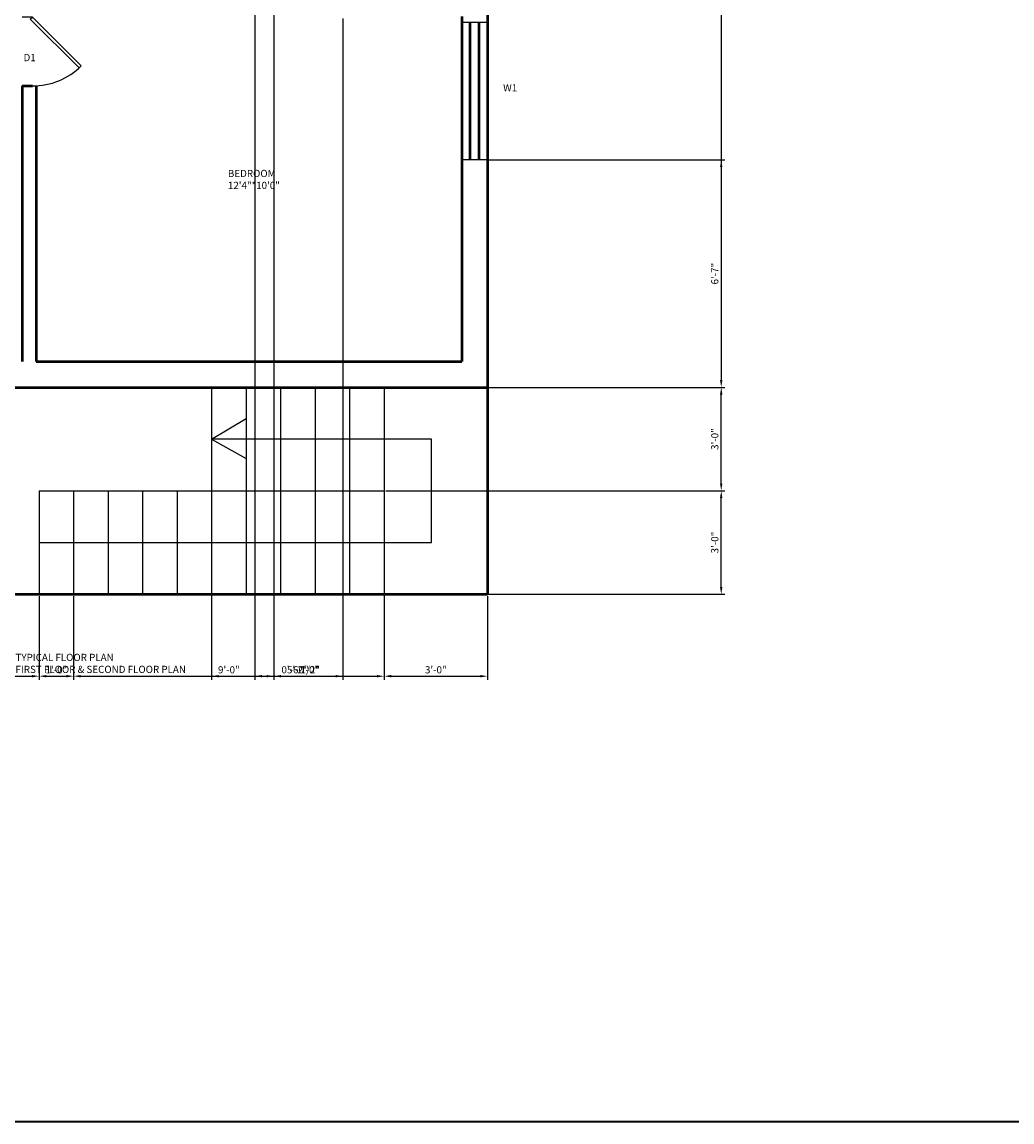
# Model space of a CAD drawing. Units: inches. Extents: x 2020 to 7901, y 1581 to 3943.
# Tile 10 of 17: x 3141 to 3486, y 1581 to 1963. Entities that reach past the tile are written whole.
import ezdxf

# ---------------------------------------------------------------- set-up
doc = ezdxf.new("R2010")
doc.units = ezdxf.units.IN
for name, color, linetype, lineweight in [('A-ANNO-DIMS', 2, 'Continuous', 18), ('A-ANNO-TEXT', 7, 'Continuous', 18), ('A-ANNO-TTLB', 7, 'Continuous', 35), ('A-AREA-IDEN', 3, 'Continuous', 18), ('A-DOOR', 4, 'Continuous', 25), ('A-FLOR-STRS', 3, 'Continuous', 25), ('A-GLAZ', 4, 'Continuous', 25), ('A-WALL', 7, 'Continuous', 50)]:
    doc.layers.add(name, color=color, linetype=linetype, lineweight=lineweight)
doc.styles.get("Standard").update_dxf_attribs({"font": 'arial.ttf'})
doc.dimstyles.new('ISO-25', dxfattribs={"dimtxt": 2.5, "dimasz": 2.5, "dimexe": 1.25, "dimexo": 0.625, "dimtad": 1, "dimdec": 1, "dimlunit": 3, "dimtxsty": 'Standard', "dimcen": 2.5, "dimadec": 0, "dimazin": 0, "dimtfac": 1, "dimtdec": 1, "dimtmove": 0, "dimatfit": 3, "dimfxl": 1, "dimarcsym": 0})

# ---------------------------------------------------------------- blocks, each defined once
blk = doc.blocks.new('*U10')
for p, q in [((0, 0), (0, -6)), ((40, 0), (40, -6))]:
    blk.add_line(p, q)
blk.add_lwpolyline([(0, 0), (28.28, 28.28), (29.52, 27.05), (1.24, -1.24)], close=True)
blk.add_arc((0, 0), 40, 0, 45)
blk = doc.blocks.new('WIN-1200')
for p, q in [((0, 9), (48, 9)), ((0, 0), (0, 9)), ((48, 9), (48, 0)), ((48, 0), (0, 0))]:
    blk.add_line(p, q)
blk = doc.blocks.new('*D50')
at = {"layer": 'A-ANNO-DIMS', "color": 0, "lineweight": -2, "transparency": 16777216}
for p, q in [((3303.94, 1915.45), (3385.87, 1915.45)), ((3384.62, 1912.95), (3384.62, 1838.84)), ((3303.94, 1836.34), (3385.87, 1836.34))]:
    blk.add_line(p, q, dxfattribs=at)
at = {"layer": 'A-ANNO-DIMS', "color": 0, "transparency": 16777216}
for points in [[(3384.2, 1912.95), (3385.03, 1912.95), (3384.62, 1915.45)], [(3384.2, 1838.84), (3385.03, 1838.84), (3384.62, 1836.34)]]:
    blk.add_solid(points, dxfattribs=at)
at = {"layer": 'DEFPOINTS', "color": 0, "transparency": 16777216}
for p in [(3303.32, 1915.45), (3303.32, 1836.34), (3384.62, 1836.34)]:
    blk.add_point(p, dxfattribs=at)
at = {"layer": 'A-ANNO-DIMS', "color": 0, "transparency": 16777216, "insert": (3382.71, 1875.9), "char_height": 2.5, "attachment_point": 5, "rotation": 90}
blk.add_mtext('6\'-7"', dxfattribs=at)
blk = doc.blocks.new('*D51')
at = {"layer": 'A-ANNO-DIMS', "color": 0, "lineweight": -2, "transparency": 16777216}
for p, q in [((2970.32, 1763.71), (2970.32, 1734.59)), ((3147.32, 1763.71), (3147.32, 1734.59)), ((2972.82, 1735.84), (3144.82, 1735.84))]:
    blk.add_line(p, q, dxfattribs=at)
at = {"layer": 'A-ANNO-DIMS', "color": 0, "transparency": 16777216}
for points in [[(2972.82, 1736.26), (2972.82, 1735.42), (2970.32, 1735.84)], [(3144.82, 1736.26), (3144.82, 1735.42), (3147.32, 1735.84)]]:
    blk.add_solid(points, dxfattribs=at)
at = {"layer": 'DEFPOINTS', "color": 0, "transparency": 16777216}
for p in [(2970.32, 1764.34), (3147.32, 1764.34), (3147.32, 1735.84)]:
    blk.add_point(p, dxfattribs=at)
at = {"layer": 'A-ANNO-DIMS', "color": 0, "transparency": 16777216, "insert": (3058.82, 1737.74), "char_height": 2.5, "attachment_point": 5}
blk.add_mtext('14\'-9"', dxfattribs=at)
blk = doc.blocks.new('*D52')
at = {"layer": 'A-ANNO-DIMS', "color": 0, "lineweight": -2, "transparency": 16777216}
for p, q in [((3147.32, 1763.71), (3147.32, 1734.59)), ((3159.32, 1763.71), (3159.32, 1734.59)), ((3149.82, 1735.84), (3156.82, 1735.84))]:
    blk.add_line(p, q, dxfattribs=at)
at = {"layer": 'A-ANNO-DIMS', "color": 0, "transparency": 16777216}
for points in [[(3149.82, 1736.26), (3149.82, 1735.42), (3147.32, 1735.84)], [(3156.82, 1736.26), (3156.82, 1735.42), (3159.32, 1735.84)]]:
    blk.add_solid(points, dxfattribs=at)
at = {"layer": 'DEFPOINTS', "color": 0, "transparency": 16777216}
for p in [(3147.32, 1764.34), (3159.32, 1764.34), (3159.32, 1735.84)]:
    blk.add_point(p, dxfattribs=at)
at = {"layer": 'A-ANNO-DIMS', "color": 0, "transparency": 16777216, "insert": (3153.32, 1737.74), "char_height": 2.5, "attachment_point": 5}
blk.add_mtext('1\'-0"', dxfattribs=at)
blk = doc.blocks.new('*D53')
at = {"layer": 'A-ANNO-DIMS', "color": 0, "lineweight": -2, "transparency": 16777216}
for p, q in [((3159.32, 1763.71), (3159.32, 1734.59)), ((3267.32, 1763.71), (3267.32, 1734.59)), ((3161.82, 1735.84), (3264.82, 1735.84))]:
    blk.add_line(p, q, dxfattribs=at)
at = {"layer": 'A-ANNO-DIMS', "color": 0, "transparency": 16777216}
for points in [[(3161.82, 1736.26), (3161.82, 1735.42), (3159.32, 1735.84)], [(3264.82, 1736.26), (3264.82, 1735.42), (3267.32, 1735.84)]]:
    blk.add_solid(points, dxfattribs=at)
at = {"layer": 'DEFPOINTS', "color": 0, "transparency": 16777216}
for p in [(3159.32, 1764.34), (3267.32, 1764.34), (3267.32, 1735.84)]:
    blk.add_point(p, dxfattribs=at)
at = {"layer": 'A-ANNO-DIMS', "color": 0, "transparency": 16777216, "insert": (3213.32, 1737.74), "char_height": 2.5, "attachment_point": 5}
blk.add_mtext('9\'-0"', dxfattribs=at)
blk = doc.blocks.new('*D54')
at = {"layer": 'A-ANNO-DIMS', "color": 0, "lineweight": -2, "transparency": 16777216}
for p, q in [((3267.32, 1763.71), (3267.32, 1734.59)), ((3303.32, 1763.71), (3303.32, 1734.59)), ((3269.82, 1735.84), (3300.82, 1735.84))]:
    blk.add_line(p, q, dxfattribs=at)
at = {"layer": 'A-ANNO-DIMS', "color": 0, "transparency": 16777216}
for points in [[(3269.82, 1736.26), (3269.82, 1735.42), (3267.32, 1735.84)], [(3300.82, 1736.26), (3300.82, 1735.42), (3303.32, 1735.84)]]:
    blk.add_solid(points, dxfattribs=at)
at = {"layer": 'DEFPOINTS', "color": 0, "transparency": 16777216}
for p in [(3267.32, 1764.34), (3303.32, 1764.34), (3303.32, 1735.84)]:
    blk.add_point(p, dxfattribs=at)
at = {"layer": 'A-ANNO-DIMS', "color": 0, "transparency": 16777216, "insert": (3285.32, 1737.74), "char_height": 2.5, "attachment_point": 5}
blk.add_mtext('3\'-0"', dxfattribs=at)
blk = doc.blocks.new('*D56')
at = {"layer": 'A-ANNO-DIMS', "color": 0, "lineweight": -2, "transparency": 16777216}
for p, q in [((3267.94, 1800.34), (3385.87, 1800.34)), ((3384.62, 1766.84), (3384.62, 1797.84)), ((3267.94, 1764.34), (3385.87, 1764.34))]:
    blk.add_line(p, q, dxfattribs=at)
at = {"layer": 'A-ANNO-DIMS', "color": 0, "transparency": 16777216}
for points in [[(3384.2, 1797.84), (3385.03, 1797.84), (3384.62, 1800.34)], [(3384.2, 1766.84), (3385.03, 1766.84), (3384.62, 1764.34)]]:
    blk.add_solid(points, dxfattribs=at)
at = {"layer": 'DEFPOINTS', "color": 0, "transparency": 16777216}
for p in [(3267.32, 1800.34), (3384.62, 1800.34), (3267.32, 1764.34)]:
    blk.add_point(p, dxfattribs=at)
at = {"layer": 'A-ANNO-DIMS', "color": 0, "transparency": 16777216, "insert": (3382.71, 1782.34), "char_height": 2.5, "attachment_point": 5, "rotation": 90}
blk.add_mtext('3\'-0"', dxfattribs=at)
blk = doc.blocks.new('*D123')
at = {"layer": 'A-ANNO-DIMS', "color": 0, "lineweight": -2, "transparency": 16777216}
for p, q in [((3303.94, 2214.34), (3385.87, 2214.34)), ((3384.62, 2211.84), (3384.62, 1838.84)), ((3303.94, 1836.34), (3385.87, 1836.34))]:
    blk.add_line(p, q, dxfattribs=at)
at = {"layer": 'A-ANNO-DIMS', "color": 0, "transparency": 16777216}
for points in [[(3384.2, 2211.84), (3385.03, 2211.84), (3384.62, 2214.34)], [(3384.2, 1838.84), (3385.03, 1838.84), (3384.62, 1836.34)]]:
    blk.add_solid(points, dxfattribs=at)
at = {"layer": 'DEFPOINTS', "color": 0, "transparency": 16777216}
for p in [(3303.32, 2214.34), (3303.32, 1836.34), (3384.62, 1836.34)]:
    blk.add_point(p, dxfattribs=at)
at = {"layer": 'A-ANNO-DIMS', "color": 0, "transparency": 16777216, "insert": (3382.71, 2025.34), "char_height": 2.5, "attachment_point": 5, "rotation": 90}
blk.add_mtext('31\'-6"', dxfattribs=at)
blk = doc.blocks.new('*D136')
at = {"layer": 'A-ANNO-DIMS', "color": 0, "lineweight": -2, "transparency": 16777216}
for p, q in [((3222.32, 1969.71), (3222.32, 1734.59)), ((3228.97, 1969.71), (3228.97, 1734.59)), ((3224.82, 1735.84), (3226.47, 1735.84)), ((3228.97, 1735.84), (3245.19, 1735.84))]:
    blk.add_line(p, q, dxfattribs=at)
at = {"layer": 'A-ANNO-DIMS', "color": 0, "transparency": 16777216}
for points in [[(3224.82, 1736.26), (3224.82, 1735.42), (3222.32, 1735.84)], [(3226.47, 1736.26), (3226.47, 1735.42), (3228.97, 1735.84)]]:
    blk.add_solid(points, dxfattribs=at)
at = {"layer": 'DEFPOINTS', "color": 0, "transparency": 16777216}
for p in [(3222.32, 1970.34), (3228.97, 1970.34), (3228.97, 1735.84)]:
    blk.add_point(p, dxfattribs=at)
at = {"layer": 'A-ANNO-DIMS', "color": 0, "transparency": 16777216, "insert": (3238.33, 1737.76), "char_height": 2.5, "attachment_point": 5}
blk.add_mtext('0\'-6 1/2"', dxfattribs=at)
blk = doc.blocks.new('*D137')
at = {"layer": 'A-ANNO-DIMS', "color": 0, "lineweight": -2, "transparency": 16777216}
for p, q in [((3228.97, 1964.72), (3228.97, 1734.59)), ((3252.97, 1964.72), (3252.97, 1734.59)), ((3231.47, 1735.84), (3250.47, 1735.84))]:
    blk.add_line(p, q, dxfattribs=at)
at = {"layer": 'A-ANNO-DIMS', "color": 0, "transparency": 16777216}
for points in [[(3231.47, 1736.26), (3231.47, 1735.42), (3228.97, 1735.84)], [(3250.47, 1736.26), (3250.47, 1735.42), (3252.97, 1735.84)]]:
    blk.add_solid(points, dxfattribs=at)
at = {"layer": 'DEFPOINTS', "color": 0, "transparency": 16777216}
for p in [(3228.97, 1965.35), (3252.97, 1965.35), (3252.97, 1735.84)]:
    blk.add_point(p, dxfattribs=at)
at = {"layer": 'A-ANNO-DIMS', "color": 0, "transparency": 16777216, "insert": (3240.97, 1737.74), "char_height": 2.5, "attachment_point": 5}
blk.add_mtext('2\'-0"', dxfattribs=at)
blk = doc.blocks.new('*D145')
at = {"layer": 'A-ANNO-DIMS', "color": 0, "lineweight": -2, "transparency": 16777216}
for p, q in [((3207.32, 1835.71), (3207.32, 1734.59)), ((3267.32, 1835.71), (3267.32, 1734.59)), ((3209.82, 1735.84), (3264.82, 1735.84))]:
    blk.add_line(p, q, dxfattribs=at)
at = {"layer": 'A-ANNO-DIMS', "color": 0, "transparency": 16777216}
for points in [[(3209.82, 1736.26), (3209.82, 1735.42), (3207.32, 1735.84)], [(3264.82, 1736.26), (3264.82, 1735.42), (3267.32, 1735.84)]]:
    blk.add_solid(points, dxfattribs=at)
at = {"layer": 'DEFPOINTS', "color": 0, "transparency": 16777216}
for p in [(3207.32, 1836.34), (3267.32, 1836.34), (3267.32, 1735.84)]:
    blk.add_point(p, dxfattribs=at)
at = {"layer": 'A-ANNO-DIMS', "color": 0, "transparency": 16777216, "insert": (3237.32, 1737.74), "char_height": 2.5, "attachment_point": 5}
blk.add_mtext('5\'-0"', dxfattribs=at)
blk = doc.blocks.new('*D146')
at = {"layer": 'A-ANNO-DIMS', "color": 0, "lineweight": -2, "transparency": 16777216}
for p, q in [((3267.94, 1836.34), (3385.87, 1836.34)), ((3384.62, 1802.84), (3384.62, 1833.84)), ((3267.94, 1800.34), (3385.87, 1800.34))]:
    blk.add_line(p, q, dxfattribs=at)
at = {"layer": 'A-ANNO-DIMS', "color": 0, "transparency": 16777216}
for points in [[(3384.2, 1833.84), (3385.03, 1833.84), (3384.62, 1836.34)], [(3384.2, 1802.84), (3385.03, 1802.84), (3384.62, 1800.34)]]:
    blk.add_solid(points, dxfattribs=at)
at = {"layer": 'DEFPOINTS', "color": 0, "transparency": 16777216}
for p in [(3267.32, 1836.34), (3384.62, 1836.34), (3267.32, 1800.34)]:
    blk.add_point(p, dxfattribs=at)
at = {"layer": 'A-ANNO-DIMS', "color": 0, "transparency": 16777216, "insert": (3382.71, 1818.34), "char_height": 2.5, "attachment_point": 5, "rotation": 90}
blk.add_mtext('3\'-0"', dxfattribs=at)

msp = doc.modelspace()

# ---------------------------------------------------------------- linework, layer by layer
at = {"layer": 'A-ANNO-TTLB'}
msp.add_lwpolyline([(2019.8, 3067.25), (4199.03, 3067.25), (4199.03, 1580.73), (2019.8, 1580.73)], close=True, dxfattribs=at)
at = {"layer": 'A-FLOR-STRS'}
for p, q in [((3207.32, 1836.34), (3207.32, 1764.34)), ((3219.32, 1836.34), (3219.32, 1764.34)), ((3231.32, 1836.34), (3231.32, 1764.34)), ((3243.32, 1836.34), (3243.32, 1764.34)), ((3255.32, 1836.34), (3255.32, 1764.34)), ((3267.32, 1836.34), (3267.32, 1764.34)), ((3207.32, 1818.34), (3219.32, 1825.47)), ((3283.87, 1818.34), (3207.32, 1818.34)), ((3207.32, 1818.34), (3219.32, 1811.61)), ((3283.87, 1782.34), (3283.87, 1818.34)), ((3147.32, 1800.34), (3147.32, 1764.34)), ((3147.32, 1800.34), (3267.32, 1800.34)), ((3159.32, 1800.34), (3159.32, 1764.34)), ((3171.32, 1800.34), (3171.32, 1764.34)), ((3183.32, 1800.34), (3183.32, 1764.34)), ((3195.32, 1800.34), (3195.32, 1764.34)), ((3147.32, 1782.34), (3283.87, 1782.34))]:
    msp.add_line(p, q, dxfattribs=at)
at = {"layer": 'A-WALL'}
for p, q in [((3303.32, 2240.34), (3303.32, 1764.34)), ((3294.32, 1965.34), (3294.32, 1845.34)), ((3297.32, 1915.45), (3297.32, 1963.45)), ((3300.32, 1963.45), (3300.32, 1915.45)), ((3141.39, 1941.19), (3144.99, 1941.19)), ((3141.39, 1941.19), (3141.39, 1845.34)), ((3146.32, 1941.23), (3146.32, 1845.34)), ((3146.32, 1845.34), (3294.32, 1845.34)), ((3061.63, 1836.34), (3303.32, 1836.34)), ((2970.32, 1764.34), (3303.32, 1764.34))]:
    msp.add_line(p, q, dxfattribs=at)

# ---------------------------------------------------------------- block references
at = {"layer": 'A-DOOR', "xscale": 0.6, "yscale": 0.6, "zscale": 0.6, "rotation": 270}
msp.add_blockref('*U10', (3144.99, 1965.19), dxfattribs=at)
at = {"layer": 'A-GLAZ', "rotation": 89.999999999998}
msp.add_blockref('WIN-1200', (3303.32, 1915.45), dxfattribs=at)

# ---------------------------------------------------------------- texts
at = {"layer": 'A-ANNO-TEXT', "char_height": 2.5, "attachment_point": 1}
for s, width, insert in [('D1', 8.3071, (3141.91, 1952.32)), ('W1', 12.448, (3308.75, 1941.8)), ('TYPICAL FLOOR PLAN\\PFIRST FLOOR & SECOND FLOOR PLAN', 248.2469, (3139.1, 1743.63))]:
    msp.add_mtext_dynamic_manual_height_columns(s, width=width, gutter_width=12.5, heights=[0], dxfattribs=dict(at, insert=insert))
at = {"layer": 'A-AREA-IDEN', "insert": (3212.99, 1912.01), "char_height": 2.5, "attachment_point": 1}
msp.add_mtext_dynamic_manual_height_columns('BEDROOM\\P12\'4"*10\'0"', width=79.8865, gutter_width=12.5, heights=[0], dxfattribs=at)

# ---------------------------------------------------------------- dimensions: what is measured, and where the dimension line sits
at = {"layer": 'A-ANNO-DIMS'}
for base, p1, p2, picture, middle in [((3384.62, 1836.34), (3303.32, 2214.34), (3303.32, 1836.34), '*D123', (3382.71, 2025.34)), ((3384.62, 1836.34), (3303.32, 1915.45), (3303.32, 1836.34), '*D50', (3382.71, 1875.9)), ((3384.62, 1836.34), (3267.32, 1800.34), (3267.32, 1836.34), '*D146', (3382.71, 1818.34)), ((3384.62, 1800.34), (3267.32, 1764.34), (3267.32, 1800.34), '*D56', (3382.71, 1782.34))]:
    dim = msp.add_linear_dim(base=base, p1=p1, p2=p2, angle=90, dimstyle='ISO-25', override={"dimdec": 1, "dimlfac": 1, "dimrnd": 0, "dimzin": 1, "dimdsep": 46, "dimlunit": 4, "dimfrac": 2}, dxfattribs=at)
    dim.commit()
    dim.dimension.update_dxf_attribs({"geometry": picture, "text_midpoint": middle})
for base, p1, p2, picture, middle in [((3228.9718, 1735.8394), (3222.3165, 1970.3394), (3228.9718, 1970.3394), '*D136', (3238.3323, 1737.7571)), ((3252.97, 1735.84), (3228.97, 1965.35), (3252.97, 1965.35), '*D137', (3240.97, 1737.74)), ((3267.32, 1735.84), (3207.32, 1836.34), (3267.32, 1836.34), '*D145', (3237.32, 1737.74)), ((3147.32, 1735.84), (2970.32, 1764.34), (3147.32, 1764.34), '*D51', (3058.82, 1737.74)), ((3159.32, 1735.84), (3147.32, 1764.34), (3159.32, 1764.34), '*D52', (3153.32, 1737.74)), ((3267.32, 1735.84), (3159.32, 1764.34), (3267.32, 1764.34), '*D53', (3213.32, 1737.74)), ((3303.32, 1735.84), (3267.32, 1764.34), (3303.32, 1764.34), '*D54', (3285.32, 1737.74))]:
    dim = msp.add_linear_dim(base=base, p1=p1, p2=p2, dimstyle='ISO-25', override={"dimdec": 1, "dimlfac": 1, "dimrnd": 0, "dimzin": 1, "dimdsep": 46, "dimlunit": 4, "dimfrac": 2}, dxfattribs=at)
    dim.commit()
    dim.dimension.update_dxf_attribs({"geometry": picture, "text_midpoint": middle})

doc.saveas('drawing.dxf')
